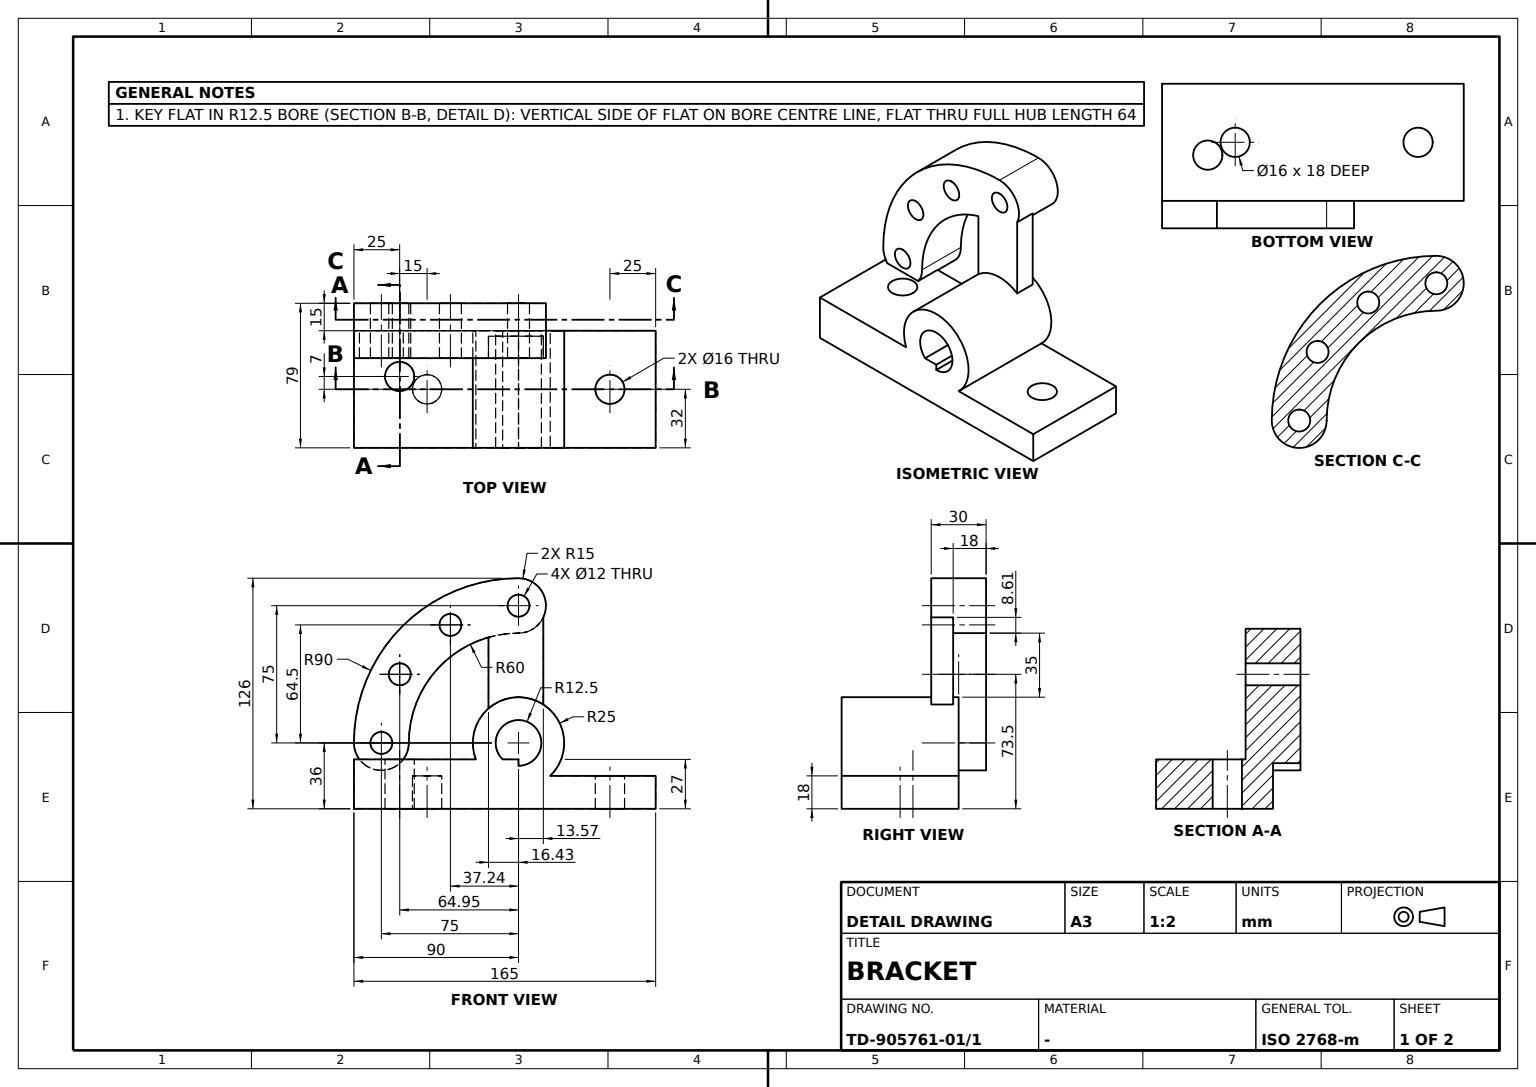
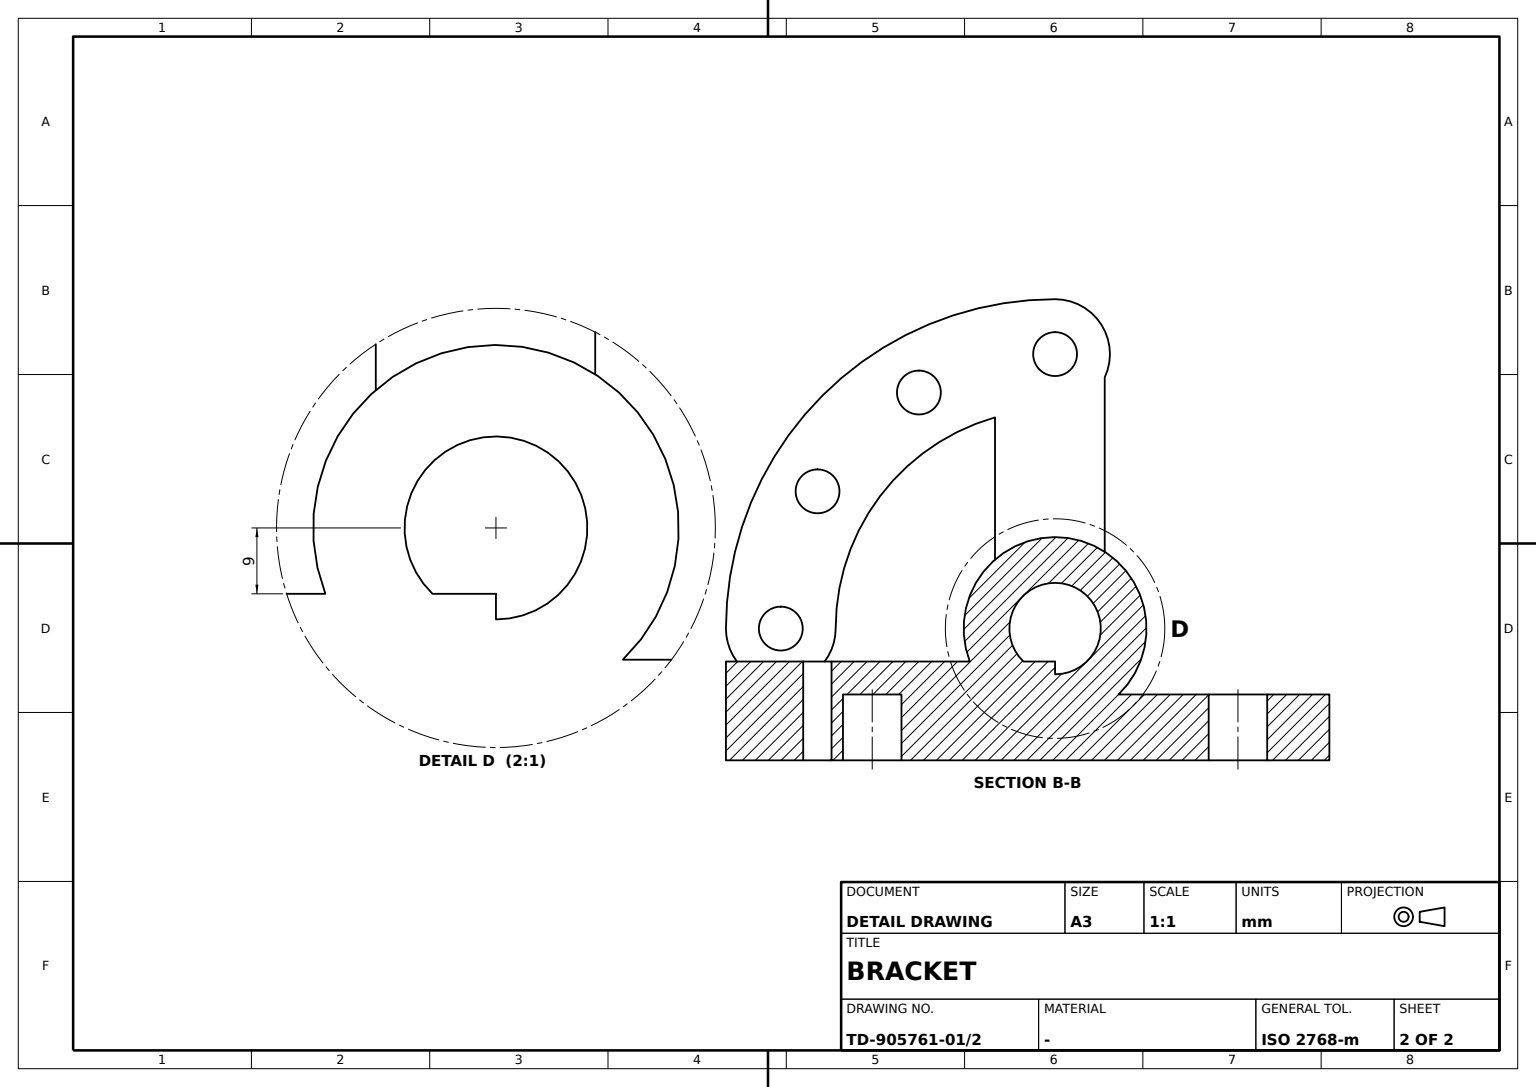
CATIA V5 part; units mm, degrees
sketch "Sketch1" plane through (0, 0, 0) normal (0, 1, 0) x (-1, 0, 0)
  circle A0 centre (0, 0) radius 12.5
  circle A1 centre (0, 0) radius 25
  dimension "radius A1" = 25
  dimension "radius A0" = 12.5
extrude "Pad1" add sketch "Sketch1" along normal mid plane 64
sketch "Sketch2" plane through (0, 0, 0) normal (0, 1, 0) x (-1, 0, 0)
  point P0 (0, -36)
  line L0 (0, -36) -> (-75, -36)
  line L1 (-75, -36) -> (-75, -18)
  line L2 (-75, -18) -> (0, -18)
  point P1 (0, -18)
  line L3 (0, -18) -> (0, -36)
  dimension "distance L3 L1" = 75
  dimension "distance L0 L2" = 18
  dimension "distance L0 x axis" = 36
  constraint coincidence P0 y-axis
  constraint coincidence P1 y-axis
  constraint horizontal L0 x-axis
  constraint horizontal L2 x-axis
  constraint vertical L1 y-axis
  constraint vertical L3 y-axis
extrude "Pad2" add sketch "Sketch2" along normal mid plane 64
sketch "Sketch3" plane through (0, 0, 0) normal (0, 1, 0) x (-1, 0, 0)
  point P0 (0, -36)
  line L0 (0, -36) -> (90, -36)
  line L1 (90, -36) -> (90, -9)
  line L2 (90, -9) -> (0, -9)
  point P1 (0, -9)
  line L3 (0, -9) -> (0, -36)
  dimension "distance L0 L2" = 27
  dimension "distance L3 L1" = 90
  dimension "distance origin L0" = 36
  constraint coincidence P0 y-axis
  constraint coincidence P1 y-axis
  constraint horizontal L0 x-axis
  constraint horizontal L2 x-axis
  constraint vertical L1 y-axis
  constraint vertical L3 y-axis
extrude "Pad3" add sketch "Sketch3" along normal mid plane 64
sketch "Sketch4" plane through (0, 32, 0) normal (0, 1, 0) x (-1, 0, 0)
  arc A0 (90, 0) -> (0, 90) centre (0, 0) ccw
  arc A1 (60, 0) -> (0, 60) centre (0, 0) ccw
  point P0 (60, 0)
  line L0 (60, 0) -> (60, 0)
  arc A2 (60, 0) -> (90, 0) centre (75, 0) ccw
  point P1 (75, 0)
  circle A3 centre (75, 0) radius 6
  point P2 (0, 0)
  circle A4 centre (64.9519, 37.5) radius 6
  point P3 (64.9519, 37.5)
  point P4 (61.646, 42.5071)
  circle A5 centre (37.2391, 64.5) radius 6
  point P5 (37.2391, 64.5)
  circle A6 centre (0, 75) radius 6
  point P6 (0, 75)
  arc A7 (0, 90) -> (0, 60) centre (0, 75) ccw
  line L1 (97.6047, 56.3521) -> (0, 0) construction
  line L2 (0, 0) -> (55.2061, 95.6198) construction
  line L3 (0, 0) -> (0, 102.3273) construction
  dimension "radius A1" = 60
  dimension "radius A2" = 15
  dimension "radius A3" = 6
  dimension "radius A4" = 6
  dimension "radius A5" = 6
  dimension "radius A6" = 6
  dimension "radius A7" = 15
  dimension "distance x axis P5" = 64.5
  dimension "distance x axis P3" = 37.5
  dimension "angle L1 L2" = 30
  dimension "angle L2 L3" = 30
  dimension "distance P5 L3" = 37.2391
  dimension "distance P3 L3" = 64.9519
  constraint coincidence P0 A1
  constraint coincidence x-axis P1
  constraint coincidence A4 P4
  constraint coincidence P6 y-axis
  constraint tangency L0 A1
  constraint tangency A2 L0
  constraint tangency A2 A0
  constraint tangency A7 A0
  constraint concentricity A2 A3
  constraint concentricity A6 A7
  constraint vertical L3 y-axis
extrude "Pad4" add sketch "Sketch4" along normal mid plane 30
sketch "Sketch5" plane through (0, 17, 0) normal (0, -1, 0) x (1, 0, 0)
  point P0 (-16.4271, 57.7074)
  line L0 (-16.4271, 57.7074) -> (-16.4271, 18.8454)
  point P1 (-16.4271, 18.8454)
  point P2 (13.5729, 68.6143)
  line L1 (13.5729, 68.6143) -> (13.5729, 20.9947)
  point P3 (13.5729, 20.9947)
  circle A0 centre (0, 0) radius 25 construction
  arc A1 (0, 60) -> (0, 90) centre (0, 75) ccw construction
  circle A2 centre (0, 0) radius 25 construction
  arc A3 (0, 60) -> (-60, 0) centre (0, 0) ccw construction
  arc A4 (0, 60) -> (13.5729, 68.6143) centre (0, 75) ccw
  point P4 (0, 60)
  arc A5 (0, 60) -> (-16.4271, 57.7074) centre (0, 0) ccw
  point P5 (0, 60)
  arc A6 (13.5729, 20.9947) -> (-16.4271, 18.8454) centre (0, 0) ccw
  dimension "distance L1 L0" = 30
  constraint vertical L0 y-axis
  constraint vertical L1 y-axis
  constraint coincidence P3 A0
  constraint coincidence P2 A1
  constraint coincidence P1 A2
  constraint coincidence P0 A3
  constraint coincidence P4 P5
extrude "Pad5" add sketch "Sketch5" against normal blind 12
sketch "Sketch6" plane through (0, 0, -18) normal (0, 0, 1) x (1, 0, 0)
  circle A0 centre (50, 0) radius 8
  point P0 (50, 0)
  line L0 (75, -32) -> (75, 32) construction
  dimension "radius A0" = 8
  dimension "distance P0 L0" = 25
  constraint coincidence P0 x-axis
extrude "Pocket1" cut sketch "Sketch6" against normal through all
mirror "Mirror1" about plane through (0, 0, 0) normal (1, 0, 0) of "Pocket1"
sketch "Sketch7" plane through (0, 0, -9) normal (0, 0, 1) x (1, 0, 0)
  circle A0 centre (-65, 7) radius 8
  point P0 (-65, 7)
  line L0 (-8.6747, 32) -> (0, 32) construction
  line L1 (-90, -32) -> (-90, 32) construction
  dimension "radius A0" = 8
  dimension "distance P0 L0" = 25
  dimension "distance P0 L1" = 25
extrude "Pocket2" cut sketch "Sketch7" against normal through all
